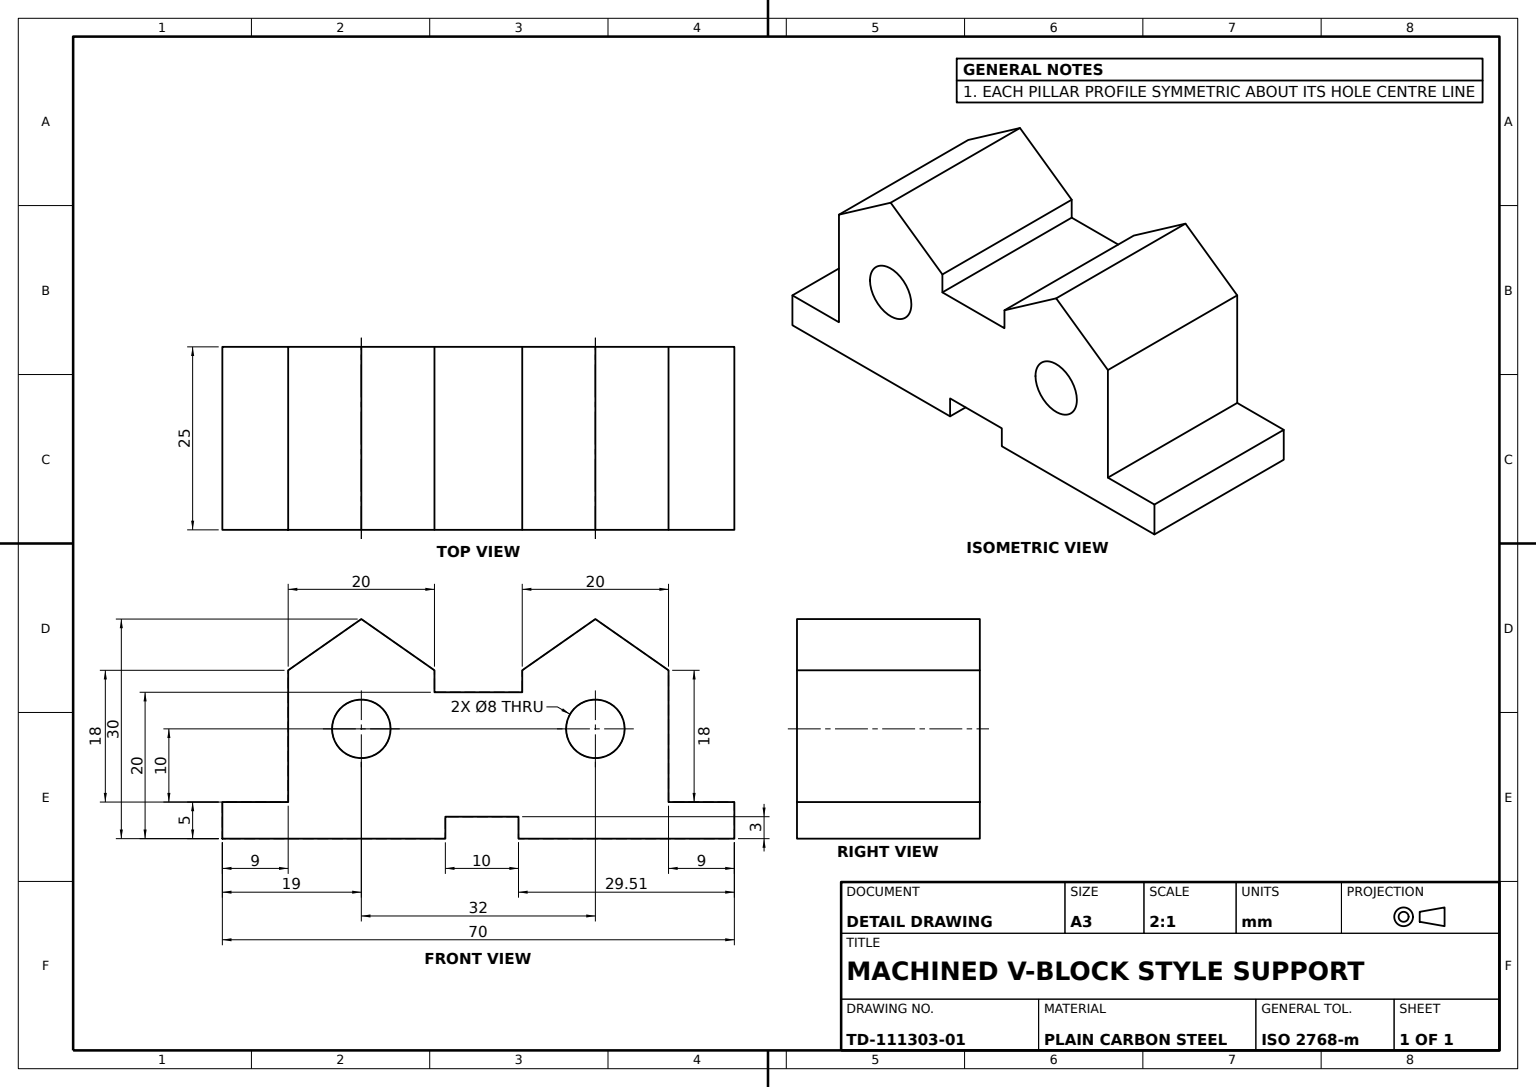
from build123d import *

# Parameters (mm, degrees)
BASE_PLATE_SKETCH_W              = 70
BASE_PLATE_SKETCH_H              = 25
BASE_PLATE_70X25X5_DEPTH         = 5
TWIN_PILLARS_DEPTH               = 25
CROSS_HOLES_SKETCH_R             = 4
CROSS_HOLES_2X_8_DEPTH           = 35
RELIEF_SLOT_SKETCH_W             = 10
RELIEF_SLOT_SKETCH_H             = 3
UNDERSIDE_RELIEF_SLOT_10X3_DEPTH = 35


with BuildPart() as part:
    # Base Plate Sketch → Base Plate 70x25x5 (new body)
    with BuildSketch(Plane(origin=(0, 0, 0), x_dir=(1, 0, 0), z_dir=(0, 1, 0))):
        with Locations((35, 12.5)):
            Rectangle(BASE_PLATE_SKETCH_W, BASE_PLATE_SKETCH_H)
    extrude(amount=BASE_PLATE_70X25X5_DEPTH)

    # Pillar Profile Sketch → Twin Pillars (add)
    with BuildSketch(Plane.XY):
        Polygon((9, 5), (9, 23), (19, 30), (29, 23), (29, 20), (41, 20), (41, 23), (51, 30), (61, 23), (61, 5), align=None)
    extrude(amount=-TWIN_PILLARS_DEPTH)

    # Cross Holes Sketch → Cross Holes 2xØ8 (cut)
    with BuildSketch(Plane.XY):
        with Locations((51, 15)):
            Circle(CROSS_HOLES_SKETCH_R)
        with Locations((19, 15)):
            Circle(CROSS_HOLES_SKETCH_R)
    extrude(amount=-CROSS_HOLES_2X_8_DEPTH, mode=Mode.SUBTRACT)

    # Relief Slot Sketch → Underside Relief Slot 10x3 (cut)
    with BuildSketch(Plane.XY):
        with Locations((35.488696345, 1.5)):
            Rectangle(RELIEF_SLOT_SKETCH_W, RELIEF_SLOT_SKETCH_H)
    extrude(amount=-UNDERSIDE_RELIEF_SLOT_10X3_DEPTH, mode=Mode.SUBTRACT)


solid = part.part
